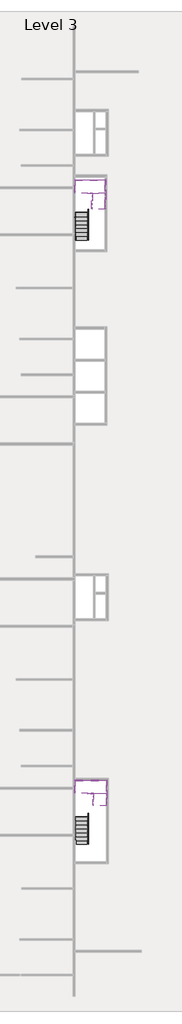
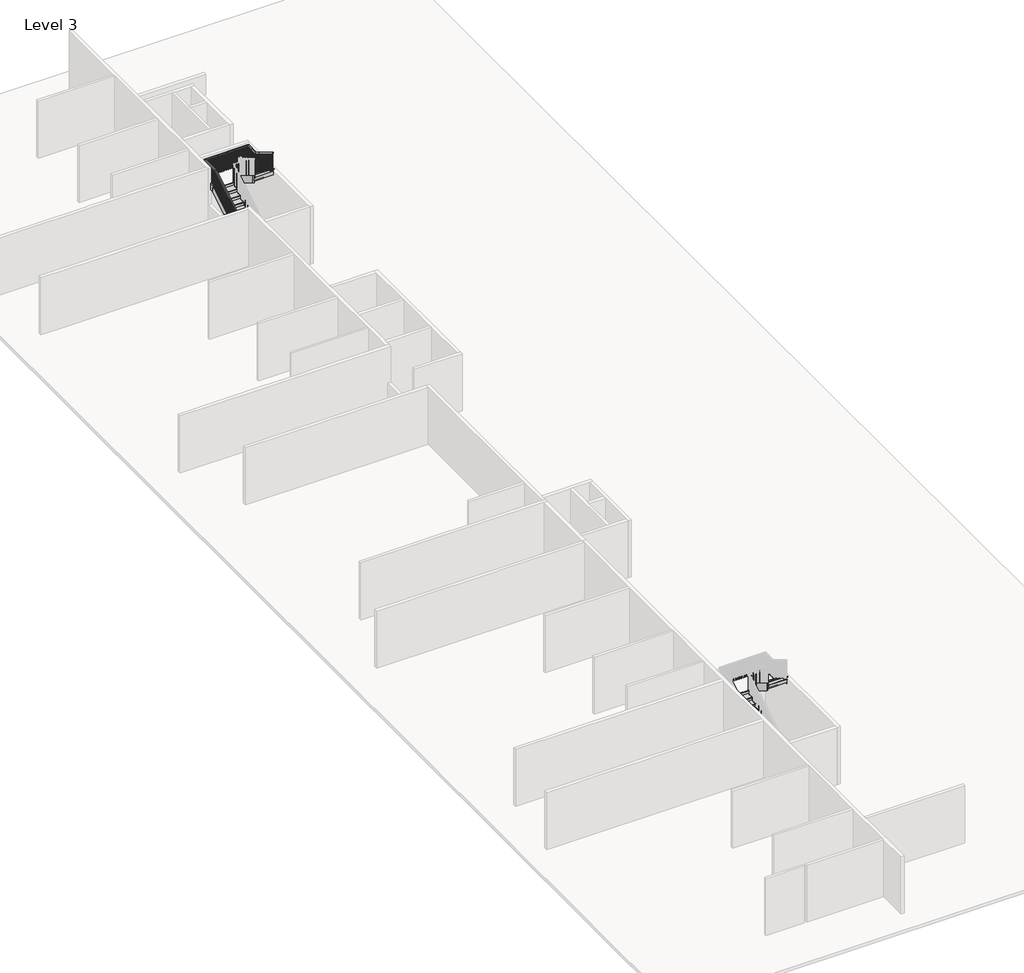
# One storey, part 8 of 8: 16 members, 4 stair flights, 2 slabs, 1 railing.
"""IFC4 building model written with IfcOpenShell, lengths in millimetres."""

from ifc_helpers import new_model, si_unit, frame, origin, place, context, project, spatial, polyline, outline, extrude, faceted_brep, transform, mapped, element, save
from components import non_monolithic_landing_2d4b1833, non_monolithic_landing_0968bfc6, stair_flight_fa816d22, stair_flight_5a0a31fc, stair_flight_0d59740e, stair_flight_4ac50f61

model = new_model("IFC4")

# Units and contexts
model_context = context("Model", 3, world=origin())
ifc_project = project(units=[si_unit("LENGTHUNIT", "METRE", prefix="MILLI")], contexts=[model_context])

# Site, building, storey
site = spatial("IfcSite", under=ifc_project)
building = spatial("IfcBuilding", under=site)
storey = spatial("IfcBuildingStorey", under=building, Name="Level 3", Elevation=31330.6172466)

# Members
placement = place(None, origin())
element("IfcMember", 1, ObjectType="Stringer - 2\" Width", at=placement, inside=storey, context=model_context, shape_type="SweptSolid", body=[
    extrude(outline(polyline([(-23154.3851539, 31330.6172466), (-23154.3851539, 31542.7317586), (-19467.0440987, 33777.4839133), (-19381.8896422, 33472.6839133), (-22916.2996422, 31330.6172466), (-23154.3851539, 31330.6172466)])), frame((-3668.2415084, 0.0, 0.0), z_axis=(1.0, 0.0, 0.0), x_axis=(0.0, 1.0, 0.0)), (0.0, 0.0, 1.0), 50.8),
])
element("IfcMember", 2, ObjectType="Stringer - 2\" Width", at=placement, inside=storey, context=model_context, shape_type="SweptSolid", body=[
    extrude(outline(polyline([(-23154.3851539, 31330.6172466), (-23154.3851539, 31542.7317586), (-19572.9851539, 33713.2772131), (-19572.9851539, 33356.8684516), (-22916.2996422, 31330.6172466), (-23154.3851539, 31330.6172466)])), frame((-2703.0415084, 0.0, 0.0), z_axis=(1.0, 0.0, 0.0), x_axis=(0.0, 1.0, 0.0)), (0.0, 0.0, 1.0), 50.8),
])
element("IfcMember", 3, ObjectType="Stringer - 2\" Width", at=placement, inside=storey, context=model_context, shape_type="SweptSolid", body=[
    extrude(outline(polyline([(-19297.9262092, 33777.4839133), (-19383.0806657, 33472.6839133), (-20360.3851539, 34064.9896637), (-20360.3851539, 34421.3984252), (-19297.9262092, 33777.4839133)])), frame((-1382.2415084, 0.0, 0.0), z_axis=(1.0, 0.0, 0.0), x_axis=(0.0, 1.0, 0.0)), (0.0, 0.0, 1.0), 50.8),
])
element("IfcMember", 4, ObjectType="Stringer - 2\" Width", at=placement, inside=storey, context=model_context, shape_type="SweptSolid", body=[
    extrude(outline(polyline([(-19522.1851539, 33913.3984252), (-19522.1851539, 33556.9896637), (-20360.3851539, 34064.9896637), (-20360.3851539, 34421.3984252), (-19522.1851539, 33913.3984252)])), frame((-2347.4415084, 0.0, 0.0), z_axis=(1.0, 0.0, 0.0), x_axis=(0.0, 1.0, 0.0)), (0.0, 0.0, 1.0), 50.8),
])
element("IfcMember", 5, ObjectType="Stringer - 2\" Width", at=placement, inside=storey, context=model_context, shape_type="Brep", body=[
    faceted_brep([(-1382.2415084, -19297.9262092, 33777.4839133), (-1331.4415084, -19297.9262092, 33777.4839133), (-1331.4415084, -18556.9851539, 33777.4839133), (-1382.2415084, -18607.7851539, 33777.4839133), (-1382.2415084, -19383.0806657, 33472.6839133), (-1382.2415084, -18607.7851539, 33472.6839133), (-1331.4415084, -19383.0806657, 33472.6839133), (-1331.4415084, -18556.9851539, 33472.6839133)], [[[0, 1, 2, 3]], [[4, 0, 3, 5]], [[6, 4, 5, 7]], [[1, 6, 7, 2]], [[1, 0, 4, 6]], [[2, 7, 5, 3]]]),
])
element("IfcMember", 6, ObjectType="Stringer - 2\" Width", at=placement, inside=storey, context=model_context, shape_type="SweptSolid", body=[
    extrude(outline(polyline([(-1331.4415084, -18556.9851539), (-1382.2415084, -18607.7851539), (-3617.4415084, -18607.7851539), (-3668.2415084, -18556.9851539), (-1331.4415084, -18556.9851539)])), frame((0.0, 0.0, 33472.6839133), z_axis=(0.0, 0.0, 1.0), x_axis=(1.0, 0.0, 0.0)), (0.0, 0.0, 1.0), 304.8),
])
element("IfcMember", 7, ObjectType="Stringer - 2\" Width", at=placement, inside=storey, context=model_context, shape_type="Brep", body=[
    faceted_brep([(-3617.4415084, -18607.7851539, 33777.4839133), (-3668.2415084, -18556.9851539, 33777.4839133), (-3668.2415084, -19467.0440987, 33777.4839133), (-3617.4415084, -19467.0440987, 33777.4839133), (-3617.4415084, -18607.7851539, 33472.6839133), (-3617.4415084, -19381.8896422, 33472.6839133), (-3668.2415084, -18556.9851539, 33472.6839133), (-3668.2415084, -19381.8896422, 33472.6839133)], [[[0, 1, 2, 3]], [[4, 0, 3, 5]], [[6, 4, 5, 7]], [[1, 6, 7, 2]], [[1, 0, 4, 6]], [[2, 7, 5, 3]]]),
])
element("IfcMember", 8, ObjectType="Stringer - 2\" Width", at=placement, inside=storey, context=model_context, shape_type="SweptSolid", body=[
    extrude(outline(polyline([(-2703.0415084, -19572.9851539), (-2703.0415084, -19522.1851539), (-2347.4415084, -19522.1851539), (-2347.4415084, -19572.9851539), (-2703.0415084, -19572.9851539)])), frame((0.0, 0.0, 33472.6839133), z_axis=(0.0, 0.0, 1.0), x_axis=(1.0, 0.0, 0.0)), (0.0, 0.0, 1.0), 304.8),
])
element("IfcMember", 9, ObjectType="Stringer - 2\" Width", at=placement, inside=storey, context=model_context, shape_type="SweptSolid", body=[
    extrude(outline(polyline([(19841.9216096, 31330.6172466), (19841.9216096, 31542.7317586), (23249.8626649, 33608.1505799), (23335.0171214, 33303.3505799), (20080.0071214, 31330.6172466), (19841.9216096, 31330.6172466)])), frame((-3668.2415084, 0.0, 0.0), z_axis=(1.0, 0.0, 0.0), x_axis=(0.0, 1.0, 0.0)), (0.0, 0.0, 1.0), 50.8),
])
element("IfcMember", 10, ObjectType="Stringer - 2\" Width", at=placement, inside=storey, context=model_context, shape_type="SweptSolid", body=[
    extrude(outline(polyline([(19841.9216096, 31330.6172466), (19841.9216096, 31542.7317586), (23143.9216096, 33543.9438798), (23143.9216096, 33187.5351183), (20080.0071214, 31330.6172466), (19841.9216096, 31330.6172466)])), frame((-2703.0415084, 0.0, 0.0), z_axis=(1.0, 0.0, 0.0), x_axis=(0.0, 1.0, 0.0)), (0.0, 0.0, 1.0), 50.8),
])
element("IfcMember", 11, ObjectType="Stringer - 2\" Width", at=placement, inside=storey, context=model_context, shape_type="SweptSolid", body=[
    extrude(outline(polyline([(23418.9805543, 33608.1505799), (23333.8260978, 33303.3505799), (22077.1216096, 34064.9896637), (22077.1216096, 34421.3984252), (23418.9805543, 33608.1505799)])), frame((-1483.8415084, 0.0, 0.0), z_axis=(1.0, 0.0, 0.0), x_axis=(0.0, 1.0, 0.0)), (0.0, 0.0, 1.0), 50.8),
])
element("IfcMember", 12, ObjectType="Stringer - 2\" Width", at=placement, inside=storey, context=model_context, shape_type="SweptSolid", body=[
    extrude(outline(polyline([(23194.7216096, 33744.0650919), (23194.7216096, 33387.6563304), (22077.1216096, 34064.9896637), (22077.1216096, 34421.3984252), (23194.7216096, 33744.0650919)])), frame((-2449.0415084, 0.0, 0.0), z_axis=(1.0, 0.0, 0.0), x_axis=(0.0, 1.0, 0.0)), (0.0, 0.0, 1.0), 50.8),
])
element("IfcMember", 13, ObjectType="Stringer - 2\" Width", at=placement, inside=storey, context=model_context, shape_type="Brep", body=[
    faceted_brep([(-1483.8415084, 23418.9805543, 33608.1505799), (-1433.0415084, 23418.9805543, 33608.1505799), (-1433.0415084, 24159.9216096, 33608.1505799), (-1483.8415084, 24109.1216096, 33608.1505799), (-1483.8415084, 23333.8260978, 33303.3505799), (-1483.8415084, 24109.1216096, 33303.3505799), (-1433.0415084, 23333.8260978, 33303.3505799), (-1433.0415084, 24159.9216096, 33303.3505799)], [[[0, 1, 2, 3]], [[4, 0, 3, 5]], [[6, 4, 5, 7]], [[1, 6, 7, 2]], [[1, 0, 4, 6]], [[2, 7, 5, 3]]]),
])
element("IfcMember", 14, ObjectType="Stringer - 2\" Width", at=placement, inside=storey, context=model_context, shape_type="SweptSolid", body=[
    extrude(outline(polyline([(-1433.0415084, 24159.9216096), (-1483.8415084, 24109.1216096), (-3617.4415084, 24109.1216096), (-3668.2415084, 24159.9216096), (-1433.0415084, 24159.9216096)])), frame((0.0, 0.0, 33303.3505799), z_axis=(0.0, 0.0, 1.0), x_axis=(1.0, 0.0, 0.0)), (0.0, 0.0, 1.0), 304.8),
])
element("IfcMember", 15, ObjectType="Stringer - 2\" Width", at=placement, inside=storey, context=model_context, shape_type="Brep", body=[
    faceted_brep([(-3617.4415084, 24109.1216096, 33608.1505799), (-3668.2415084, 24159.9216096, 33608.1505799), (-3668.2415084, 23249.8626649, 33608.1505799), (-3617.4415084, 23249.8626649, 33608.1505799), (-3617.4415084, 24109.1216096, 33303.3505799), (-3617.4415084, 23335.0171214, 33303.3505799), (-3668.2415084, 24159.9216096, 33303.3505799), (-3668.2415084, 23335.0171214, 33303.3505799)], [[[0, 1, 2, 3]], [[4, 0, 3, 5]], [[6, 4, 5, 7]], [[1, 6, 7, 2]], [[1, 0, 4, 6]], [[2, 7, 5, 3]]]),
])
element("IfcMember", 16, ObjectType="Stringer - 2\" Width", at=placement, inside=storey, context=model_context, shape_type="SweptSolid", body=[
    extrude(outline(polyline([(-2703.0415084, 23143.9216096), (-2703.0415084, 23194.7216096), (-2449.0415084, 23194.7216096), (-2449.0415084, 23143.9216096), (-2703.0415084, 23143.9216096)])), frame((0.0, 0.0, 33303.3505799), z_axis=(0.0, 0.0, 1.0), x_axis=(1.0, 0.0, 0.0)), (0.0, 0.0, 1.0), 304.8),
])

# Railing
element("IfcRailing", 17, ObjectType="Handrail - Rectangular", at=placement, inside=storey, context=model_context, shape_type="SolidModel", body=[
    faceted_brep([(-3617.4415084, 19841.9216096, 32414.3505799), (-3617.4415084, 19841.9216096, 32354.9491197), (-3566.6415084, 19841.9216096, 32354.9491197), (-3566.6415084, 19841.9216096, 32414.3505799), (-3617.4415084, 23194.7216096, 34446.3505799), (-3617.4415084, 23208.914019, 34395.5505799), (-3566.6415084, 23208.914019, 34395.5505799), (-3566.6415084, 23194.7216096, 34446.3505799), (-3617.4415084, 24109.1216096, 34446.3505799), (-3617.4415084, 24109.1216096, 34395.5505799), (-3566.6415084, 24058.3216096, 34395.5505799), (-3566.6415084, 24058.3216096, 34446.3505799), (-1483.8415084, 24109.1216096, 34446.3505799), (-1483.8415084, 24109.1216096, 34395.5505799), (-1534.6415084, 24058.3216096, 34395.5505799), (-1534.6415084, 24058.3216096, 34446.3505799), (-1483.8415084, 23474.1216096, 34446.3505799), (-1483.8415084, 23459.9292002, 34395.5505799), (-1534.6415084, 23459.9292002, 34395.5505799), (-1534.6415084, 23474.1216096, 34446.3505799), (-1483.8415084, 23194.7216096, 34615.6839133), (-1483.8415084, 23168.3918824, 34572.2398634), (-1534.6415084, 23168.3918824, 34572.2398634), (-1534.6415084, 23194.7216096, 34615.6839133), (-1483.8415084, 22077.1216096, 35293.0172466), (-1534.6415084, 22077.1216096, 35293.0172466), (-1534.6415084, 22077.1216096, 35233.6157863), (-1483.8415084, 22077.1216096, 35233.6157863)], [[[0, 1, 2, 3]], [[1, 0, 4, 5]], [[2, 1, 5, 6]], [[3, 2, 6, 7]], [[0, 3, 7, 4]], [[5, 4, 8, 9]], [[6, 5, 9, 10]], [[7, 6, 10, 11]], [[4, 7, 11, 8]], [[9, 8, 12, 13]], [[10, 9, 13, 14]], [[11, 10, 14, 15]], [[8, 11, 15, 12]], [[13, 12, 16, 17]], [[14, 13, 17, 18]], [[15, 14, 18, 19]], [[12, 15, 19, 16]], [[17, 16, 20, 21]], [[18, 17, 21, 22]], [[19, 18, 22, 23]], [[16, 19, 23, 20]], [[24, 25, 26, 27]], [[21, 20, 24, 27]], [[22, 21, 27, 26]], [[23, 22, 26, 25]], [[20, 23, 25, 24]]]),
    extrude(outline(polyline([(22188.2466096, 35166.2673015), (22188.2466096, 34209.2839133), (22169.1966096, 34209.2839133), (22169.1966096, 35177.812756), (22188.2466096, 35166.2673015)])), frame((-1518.7665084, 0.0, 0.0), z_axis=(1.0, 0.0, 0.0), x_axis=(0.0, 1.0, 0.0)), (0.0, 0.0, 1.0), 19.05),
    extrude(outline(polyline([(22289.8466096, 35104.6915439), (22289.8466096, 34209.2839133), (22270.7966096, 34209.2839133), (22270.7966096, 35116.2369985), (22289.8466096, 35104.6915439)])), frame((-1518.7665084, 0.0, 0.0), z_axis=(1.0, 0.0, 0.0), x_axis=(0.0, 1.0, 0.0)), (0.0, 0.0, 1.0), 19.05),
    extrude(outline(polyline([(22391.4466096, 35043.1157863), (22391.4466096, 34039.9505799), (22372.3966096, 34039.9505799), (22372.3966096, 35054.6612409), (22391.4466096, 35043.1157863)])), frame((-1518.7665084, 0.0, 0.0), z_axis=(1.0, 0.0, 0.0), x_axis=(0.0, 1.0, 0.0)), (0.0, 0.0, 1.0), 19.05),
    extrude(outline(polyline([(22493.0466096, 34981.5400288), (22493.0466096, 34039.9505799), (22473.9966096, 34039.9505799), (22473.9966096, 34993.0854833), (22493.0466096, 34981.5400288)])), frame((-1518.7665084, 0.0, 0.0), z_axis=(1.0, 0.0, 0.0), x_axis=(0.0, 1.0, 0.0)), (0.0, 0.0, 1.0), 19.05),
    extrude(outline(polyline([(22594.6466096, 34919.9642712), (22594.6466096, 34039.9505799), (22575.5966096, 34039.9505799), (22575.5966096, 34931.5097257), (22594.6466096, 34919.9642712)])), frame((-1518.7665084, 0.0, 0.0), z_axis=(1.0, 0.0, 0.0), x_axis=(0.0, 1.0, 0.0)), (0.0, 0.0, 1.0), 19.05),
    extrude(outline(polyline([(22696.2466096, 34858.3885136), (22696.2466096, 33870.6172466), (22677.1966096, 33870.6172466), (22677.1966096, 34869.9339682), (22696.2466096, 34858.3885136)])), frame((-1518.7665084, 0.0, 0.0), z_axis=(1.0, 0.0, 0.0), x_axis=(0.0, 1.0, 0.0)), (0.0, 0.0, 1.0), 19.05),
    extrude(outline(polyline([(22797.8466096, 34796.812756), (22797.8466096, 33870.6172466), (22778.7966096, 33870.6172466), (22778.7966096, 34808.3582106), (22797.8466096, 34796.812756)])), frame((-1518.7665084, 0.0, 0.0), z_axis=(1.0, 0.0, 0.0), x_axis=(0.0, 1.0, 0.0)), (0.0, 0.0, 1.0), 19.05),
    extrude(outline(polyline([(22899.4466096, 34735.2369985), (22899.4466096, 33870.6172466), (22880.3966096, 33870.6172466), (22880.3966096, 34746.782453), (22899.4466096, 34735.2369985)])), frame((-1518.7665084, 0.0, 0.0), z_axis=(1.0, 0.0, 0.0), x_axis=(0.0, 1.0, 0.0)), (0.0, 0.0, 1.0), 19.05),
    extrude(outline(polyline([(23001.0466096, 34673.6612409), (23001.0466096, 33701.2839133), (22981.9966096, 33701.2839133), (22981.9966096, 34685.2066954), (23001.0466096, 34673.6612409)])), frame((-1518.7665084, 0.0, 0.0), z_axis=(1.0, 0.0, 0.0), x_axis=(0.0, 1.0, 0.0)), (0.0, 0.0, 1.0), 19.05),
    extrude(outline(polyline([(23102.6466096, 34612.0854833), (23102.6466096, 33701.2839133), (23083.5966096, 33701.2839133), (23083.5966096, 34623.6309379), (23102.6466096, 34612.0854833)])), frame((-1518.7665084, 0.0, 0.0), z_axis=(1.0, 0.0, 0.0), x_axis=(0.0, 1.0, 0.0)), (0.0, 0.0, 1.0), 19.05),
    extrude(outline(polyline([(23280.4466096, 34504.3279076), (23280.4466096, 33531.9505799), (23261.3966096, 33531.9505799), (23261.3966096, 34515.8733621), (23280.4466096, 34504.3279076)])), frame((-1518.7665084, 0.0, 0.0), z_axis=(1.0, 0.0, 0.0), x_axis=(0.0, 1.0, 0.0)), (0.0, 0.0, 1.0), 19.05),
    extrude(outline(polyline([(23382.0466096, 34442.75215), (23382.0466096, 33531.9505799), (23362.9966096, 33531.9505799), (23362.9966096, 34454.2976045), (23382.0466096, 34442.75215)])), frame((-1518.7665084, 0.0, 0.0), z_axis=(1.0, 0.0, 0.0), x_axis=(0.0, 1.0, 0.0)), (0.0, 0.0, 1.0), 19.05),
    extrude(outline(polyline([(-1499.7165084, 23483.6466096), (-1499.7165084, 23464.5966096), (-1518.7665084, 23464.5966096), (-1518.7665084, 23483.6466096), (-1499.7165084, 23483.6466096)])), frame((0.0, 0.0, 33531.9505799), z_axis=(0.0, 0.0, 1.0), x_axis=(1.0, 0.0, 0.0)), (0.0, 0.0, 1.0), 863.6),
    extrude(outline(polyline([(-1499.7165084, 23585.2466096), (-1499.7165084, 23566.1966096), (-1518.7665084, 23566.1966096), (-1518.7665084, 23585.2466096), (-1499.7165084, 23585.2466096)])), frame((0.0, 0.0, 33531.9505799), z_axis=(0.0, 0.0, 1.0), x_axis=(1.0, 0.0, 0.0)), (0.0, 0.0, 1.0), 863.6),
    extrude(outline(polyline([(-1499.7165084, 23686.8466096), (-1499.7165084, 23667.7966096), (-1518.7665084, 23667.7966096), (-1518.7665084, 23686.8466096), (-1499.7165084, 23686.8466096)])), frame((0.0, 0.0, 33531.9505799), z_axis=(0.0, 0.0, 1.0), x_axis=(1.0, 0.0, 0.0)), (0.0, 0.0, 1.0), 863.6),
    extrude(outline(polyline([(-1499.7165084, 23788.4466096), (-1499.7165084, 23769.3966096), (-1518.7665084, 23769.3966096), (-1518.7665084, 23788.4466096), (-1499.7165084, 23788.4466096)])), frame((0.0, 0.0, 33531.9505799), z_axis=(0.0, 0.0, 1.0), x_axis=(1.0, 0.0, 0.0)), (0.0, 0.0, 1.0), 863.6),
    extrude(outline(polyline([(-1499.7165084, 23890.0466096), (-1499.7165084, 23870.9966096), (-1518.7665084, 23870.9966096), (-1518.7665084, 23890.0466096), (-1499.7165084, 23890.0466096)])), frame((0.0, 0.0, 33531.9505799), z_axis=(0.0, 0.0, 1.0), x_axis=(1.0, 0.0, 0.0)), (0.0, 0.0, 1.0), 863.6),
    extrude(outline(polyline([(-1499.7165084, 23991.6466096), (-1499.7165084, 23972.5966096), (-1518.7665084, 23972.5966096), (-1518.7665084, 23991.6466096), (-1499.7165084, 23991.6466096)])), frame((0.0, 0.0, 33531.9505799), z_axis=(0.0, 0.0, 1.0), x_axis=(1.0, 0.0, 0.0)), (0.0, 0.0, 1.0), 863.6),
    extrude(outline(polyline([(-1569.5665084, 24093.2466096), (-1550.5165084, 24093.2466096), (-1550.5165084, 24074.1966096), (-1569.5665084, 24074.1966096), (-1569.5665084, 24093.2466096)])), frame((0.0, 0.0, 33531.9505799), z_axis=(0.0, 0.0, 1.0), x_axis=(1.0, 0.0, 0.0)), (0.0, 0.0, 1.0), 863.6),
    extrude(outline(polyline([(-1671.1665084, 24093.2466096), (-1652.1165084, 24093.2466096), (-1652.1165084, 24074.1966096), (-1671.1665084, 24074.1966096), (-1671.1665084, 24093.2466096)])), frame((0.0, 0.0, 33531.9505799), z_axis=(0.0, 0.0, 1.0), x_axis=(1.0, 0.0, 0.0)), (0.0, 0.0, 1.0), 863.6),
    extrude(outline(polyline([(-1772.7665084, 24093.2466096), (-1753.7165084, 24093.2466096), (-1753.7165084, 24074.1966096), (-1772.7665084, 24074.1966096), (-1772.7665084, 24093.2466096)])), frame((0.0, 0.0, 33531.9505799), z_axis=(0.0, 0.0, 1.0), x_axis=(1.0, 0.0, 0.0)), (0.0, 0.0, 1.0), 863.6),
    extrude(outline(polyline([(-1874.3665084, 24093.2466096), (-1855.3165084, 24093.2466096), (-1855.3165084, 24074.1966096), (-1874.3665084, 24074.1966096), (-1874.3665084, 24093.2466096)])), frame((0.0, 0.0, 33531.9505799), z_axis=(0.0, 0.0, 1.0), x_axis=(1.0, 0.0, 0.0)), (0.0, 0.0, 1.0), 863.6),
    extrude(outline(polyline([(-1975.9665084, 24093.2466096), (-1956.9165084, 24093.2466096), (-1956.9165084, 24074.1966096), (-1975.9665084, 24074.1966096), (-1975.9665084, 24093.2466096)])), frame((0.0, 0.0, 33531.9505799), z_axis=(0.0, 0.0, 1.0), x_axis=(1.0, 0.0, 0.0)), (0.0, 0.0, 1.0), 863.6),
    extrude(outline(polyline([(-2077.5665084, 24093.2466096), (-2058.5165084, 24093.2466096), (-2058.5165084, 24074.1966096), (-2077.5665084, 24074.1966096), (-2077.5665084, 24093.2466096)])), frame((0.0, 0.0, 33531.9505799), z_axis=(0.0, 0.0, 1.0), x_axis=(1.0, 0.0, 0.0)), (0.0, 0.0, 1.0), 863.6),
    extrude(outline(polyline([(-2179.1665084, 24093.2466096), (-2160.1165084, 24093.2466096), (-2160.1165084, 24074.1966096), (-2179.1665084, 24074.1966096), (-2179.1665084, 24093.2466096)])), frame((0.0, 0.0, 33531.9505799), z_axis=(0.0, 0.0, 1.0), x_axis=(1.0, 0.0, 0.0)), (0.0, 0.0, 1.0), 863.6),
    extrude(outline(polyline([(-2280.7665084, 24093.2466096), (-2261.7165084, 24093.2466096), (-2261.7165084, 24074.1966096), (-2280.7665084, 24074.1966096), (-2280.7665084, 24093.2466096)])), frame((0.0, 0.0, 33531.9505799), z_axis=(0.0, 0.0, 1.0), x_axis=(1.0, 0.0, 0.0)), (0.0, 0.0, 1.0), 863.6),
    extrude(outline(polyline([(-2382.3665084, 24093.2466096), (-2363.3165084, 24093.2466096), (-2363.3165084, 24074.1966096), (-2382.3665084, 24074.1966096), (-2382.3665084, 24093.2466096)])), frame((0.0, 0.0, 33531.9505799), z_axis=(0.0, 0.0, 1.0), x_axis=(1.0, 0.0, 0.0)), (0.0, 0.0, 1.0), 863.6),
    extrude(outline(polyline([(-2483.9665084, 24093.2466096), (-2464.9165084, 24093.2466096), (-2464.9165084, 24074.1966096), (-2483.9665084, 24074.1966096), (-2483.9665084, 24093.2466096)])), frame((0.0, 0.0, 33531.9505799), z_axis=(0.0, 0.0, 1.0), x_axis=(1.0, 0.0, 0.0)), (0.0, 0.0, 1.0), 863.6),
    extrude(outline(polyline([(-2585.5665084, 24093.2466096), (-2566.5165084, 24093.2466096), (-2566.5165084, 24074.1966096), (-2585.5665084, 24074.1966096), (-2585.5665084, 24093.2466096)])), frame((0.0, 0.0, 33531.9505799), z_axis=(0.0, 0.0, 1.0), x_axis=(1.0, 0.0, 0.0)), (0.0, 0.0, 1.0), 863.6),
    extrude(outline(polyline([(-2687.1665084, 24093.2466096), (-2668.1165084, 24093.2466096), (-2668.1165084, 24074.1966096), (-2687.1665084, 24074.1966096), (-2687.1665084, 24093.2466096)])), frame((0.0, 0.0, 33531.9505799), z_axis=(0.0, 0.0, 1.0), x_axis=(1.0, 0.0, 0.0)), (0.0, 0.0, 1.0), 863.6),
    extrude(outline(polyline([(-2788.7665084, 24093.2466096), (-2769.7165084, 24093.2466096), (-2769.7165084, 24074.1966096), (-2788.7665084, 24074.1966096), (-2788.7665084, 24093.2466096)])), frame((0.0, 0.0, 33531.9505799), z_axis=(0.0, 0.0, 1.0), x_axis=(1.0, 0.0, 0.0)), (0.0, 0.0, 1.0), 863.6),
    extrude(outline(polyline([(-2890.3665084, 24093.2466096), (-2871.3165084, 24093.2466096), (-2871.3165084, 24074.1966096), (-2890.3665084, 24074.1966096), (-2890.3665084, 24093.2466096)])), frame((0.0, 0.0, 33531.9505799), z_axis=(0.0, 0.0, 1.0), x_axis=(1.0, 0.0, 0.0)), (0.0, 0.0, 1.0), 863.6),
    extrude(outline(polyline([(-2991.9665084, 24093.2466096), (-2972.9165084, 24093.2466096), (-2972.9165084, 24074.1966096), (-2991.9665084, 24074.1966096), (-2991.9665084, 24093.2466096)])), frame((0.0, 0.0, 33531.9505799), z_axis=(0.0, 0.0, 1.0), x_axis=(1.0, 0.0, 0.0)), (0.0, 0.0, 1.0), 863.6),
    extrude(outline(polyline([(-3093.5665084, 24093.2466096), (-3074.5165084, 24093.2466096), (-3074.5165084, 24074.1966096), (-3093.5665084, 24074.1966096), (-3093.5665084, 24093.2466096)])), frame((0.0, 0.0, 33531.9505799), z_axis=(0.0, 0.0, 1.0), x_axis=(1.0, 0.0, 0.0)), (0.0, 0.0, 1.0), 863.6),
    extrude(outline(polyline([(-3195.1665084, 24093.2466096), (-3176.1165084, 24093.2466096), (-3176.1165084, 24074.1966096), (-3195.1665084, 24074.1966096), (-3195.1665084, 24093.2466096)])), frame((0.0, 0.0, 33531.9505799), z_axis=(0.0, 0.0, 1.0), x_axis=(1.0, 0.0, 0.0)), (0.0, 0.0, 1.0), 863.6),
    extrude(outline(polyline([(-3296.7665084, 24093.2466096), (-3277.7165084, 24093.2466096), (-3277.7165084, 24074.1966096), (-3296.7665084, 24074.1966096), (-3296.7665084, 24093.2466096)])), frame((0.0, 0.0, 33531.9505799), z_axis=(0.0, 0.0, 1.0), x_axis=(1.0, 0.0, 0.0)), (0.0, 0.0, 1.0), 863.6),
    extrude(outline(polyline([(-3398.3665084, 24093.2466096), (-3379.3165084, 24093.2466096), (-3379.3165084, 24074.1966096), (-3398.3665084, 24074.1966096), (-3398.3665084, 24093.2466096)])), frame((0.0, 0.0, 33531.9505799), z_axis=(0.0, 0.0, 1.0), x_axis=(1.0, 0.0, 0.0)), (0.0, 0.0, 1.0), 863.6),
    extrude(outline(polyline([(-3499.9665084, 24093.2466096), (-3480.9165084, 24093.2466096), (-3480.9165084, 24074.1966096), (-3499.9665084, 24074.1966096), (-3499.9665084, 24093.2466096)])), frame((0.0, 0.0, 33531.9505799), z_axis=(0.0, 0.0, 1.0), x_axis=(1.0, 0.0, 0.0)), (0.0, 0.0, 1.0), 863.6),
    extrude(outline(polyline([(-3601.5665084, 23997.9966096), (-3601.5665084, 24017.0466096), (-3582.5165084, 24017.0466096), (-3582.5165084, 23997.9966096), (-3601.5665084, 23997.9966096)])), frame((0.0, 0.0, 33531.9505799), z_axis=(0.0, 0.0, 1.0), x_axis=(1.0, 0.0, 0.0)), (0.0, 0.0, 1.0), 863.6),
    extrude(outline(polyline([(-3601.5665084, 23896.3966096), (-3601.5665084, 23915.4466096), (-3582.5165084, 23915.4466096), (-3582.5165084, 23896.3966096), (-3601.5665084, 23896.3966096)])), frame((0.0, 0.0, 33531.9505799), z_axis=(0.0, 0.0, 1.0), x_axis=(1.0, 0.0, 0.0)), (0.0, 0.0, 1.0), 863.6),
    extrude(outline(polyline([(-3601.5665084, 23794.7966096), (-3601.5665084, 23813.8466096), (-3582.5165084, 23813.8466096), (-3582.5165084, 23794.7966096), (-3601.5665084, 23794.7966096)])), frame((0.0, 0.0, 33531.9505799), z_axis=(0.0, 0.0, 1.0), x_axis=(1.0, 0.0, 0.0)), (0.0, 0.0, 1.0), 863.6),
    extrude(outline(polyline([(-3601.5665084, 23693.1966096), (-3601.5665084, 23712.2466096), (-3582.5165084, 23712.2466096), (-3582.5165084, 23693.1966096), (-3601.5665084, 23693.1966096)])), frame((0.0, 0.0, 33531.9505799), z_axis=(0.0, 0.0, 1.0), x_axis=(1.0, 0.0, 0.0)), (0.0, 0.0, 1.0), 863.6),
    extrude(outline(polyline([(-3601.5665084, 23591.5966096), (-3601.5665084, 23610.6466096), (-3582.5165084, 23610.6466096), (-3582.5165084, 23591.5966096), (-3601.5665084, 23591.5966096)])), frame((0.0, 0.0, 33531.9505799), z_axis=(0.0, 0.0, 1.0), x_axis=(1.0, 0.0, 0.0)), (0.0, 0.0, 1.0), 863.6),
    extrude(outline(polyline([(-3601.5665084, 23489.9966096), (-3601.5665084, 23509.0466096), (-3582.5165084, 23509.0466096), (-3582.5165084, 23489.9966096), (-3601.5665084, 23489.9966096)])), frame((0.0, 0.0, 33531.9505799), z_axis=(0.0, 0.0, 1.0), x_axis=(1.0, 0.0, 0.0)), (0.0, 0.0, 1.0), 863.6),
    extrude(outline(polyline([(-3601.5665084, 23388.3966096), (-3601.5665084, 23407.4466096), (-3582.5165084, 23407.4466096), (-3582.5165084, 23388.3966096), (-3601.5665084, 23388.3966096)])), frame((0.0, 0.0, 33531.9505799), z_axis=(0.0, 0.0, 1.0), x_axis=(1.0, 0.0, 0.0)), (0.0, 0.0, 1.0), 863.6),
    extrude(outline(polyline([(-3601.5665084, 23286.7966096), (-3601.5665084, 23305.8466096), (-3582.5165084, 23305.8466096), (-3582.5165084, 23286.7966096), (-3601.5665084, 23286.7966096)])), frame((0.0, 0.0, 33531.9505799), z_axis=(0.0, 0.0, 1.0), x_axis=(1.0, 0.0, 0.0)), (0.0, 0.0, 1.0), 863.6),
    extrude(outline(polyline([(23102.6466096, 34331.1460894), (23102.6466096, 33362.6172466), (23083.5966096, 33362.6172466), (23083.5966096, 34319.6006348), (23102.6466096, 34331.1460894)])), frame((-3601.5665084, 0.0, 0.0), z_axis=(1.0, 0.0, 0.0), x_axis=(0.0, 1.0, 0.0)), (0.0, 0.0, 1.0), 19.05),
    extrude(outline(polyline([(23001.0466096, 34269.5703318), (23001.0466096, 33362.6172466), (22981.9966096, 33362.6172466), (22981.9966096, 34258.0248773), (23001.0466096, 34269.5703318)])), frame((-3601.5665084, 0.0, 0.0), z_axis=(1.0, 0.0, 0.0), x_axis=(0.0, 1.0, 0.0)), (0.0, 0.0, 1.0), 19.05),
    extrude(outline(polyline([(22899.4466096, 34207.9945742), (22899.4466096, 33193.2839133), (22880.3966096, 33193.2839133), (22880.3966096, 34196.4491197), (22899.4466096, 34207.9945742)])), frame((-3601.5665084, 0.0, 0.0), z_axis=(1.0, 0.0, 0.0), x_axis=(0.0, 1.0, 0.0)), (0.0, 0.0, 1.0), 19.05),
    extrude(outline(polyline([(22797.8466096, 34146.4188166), (22797.8466096, 33193.2839133), (22778.7966096, 33193.2839133), (22778.7966096, 34134.8733621), (22797.8466096, 34146.4188166)])), frame((-3601.5665084, 0.0, 0.0), z_axis=(1.0, 0.0, 0.0), x_axis=(0.0, 1.0, 0.0)), (0.0, 0.0, 1.0), 19.05),
    extrude(outline(polyline([(22696.2466096, 34084.8430591), (22696.2466096, 33193.2839133), (22677.1966096, 33193.2839133), (22677.1966096, 34073.2976045), (22696.2466096, 34084.8430591)])), frame((-3601.5665084, 0.0, 0.0), z_axis=(1.0, 0.0, 0.0), x_axis=(0.0, 1.0, 0.0)), (0.0, 0.0, 1.0), 19.05),
    extrude(outline(polyline([(22594.6466096, 34023.2673015), (22594.6466096, 33023.9505799), (22575.5966096, 33023.9505799), (22575.5966096, 34011.721847), (22594.6466096, 34023.2673015)])), frame((-3601.5665084, 0.0, 0.0), z_axis=(1.0, 0.0, 0.0), x_axis=(0.0, 1.0, 0.0)), (0.0, 0.0, 1.0), 19.05),
    extrude(outline(polyline([(22493.0466096, 33961.6915439), (22493.0466096, 33023.9505799), (22473.9966096, 33023.9505799), (22473.9966096, 33950.1460894), (22493.0466096, 33961.6915439)])), frame((-3601.5665084, 0.0, 0.0), z_axis=(1.0, 0.0, 0.0), x_axis=(0.0, 1.0, 0.0)), (0.0, 0.0, 1.0), 19.05),
    extrude(outline(polyline([(22391.4466096, 33900.1157863), (22391.4466096, 33023.9505799), (22372.3966096, 33023.9505799), (22372.3966096, 33888.5703318), (22391.4466096, 33900.1157863)])), frame((-3601.5665084, 0.0, 0.0), z_axis=(1.0, 0.0, 0.0), x_axis=(0.0, 1.0, 0.0)), (0.0, 0.0, 1.0), 19.05),
    extrude(outline(polyline([(22289.8466096, 33838.5400288), (22289.8466096, 32854.6172466), (22270.7966096, 32854.6172466), (22270.7966096, 33826.9945742), (22289.8466096, 33838.5400288)])), frame((-3601.5665084, 0.0, 0.0), z_axis=(1.0, 0.0, 0.0), x_axis=(0.0, 1.0, 0.0)), (0.0, 0.0, 1.0), 19.05),
    extrude(outline(polyline([(22188.2466096, 33776.9642712), (22188.2466096, 32854.6172466), (22169.1966096, 32854.6172466), (22169.1966096, 33765.4188166), (22188.2466096, 33776.9642712)])), frame((-3601.5665084, 0.0, 0.0), z_axis=(1.0, 0.0, 0.0), x_axis=(0.0, 1.0, 0.0)), (0.0, 0.0, 1.0), 19.05),
    extrude(outline(polyline([(22086.6466096, 33715.3885136), (22086.6466096, 32854.6172466), (22067.5966096, 32854.6172466), (22067.5966096, 33703.8430591), (22086.6466096, 33715.3885136)])), frame((-3601.5665084, 0.0, 0.0), z_axis=(1.0, 0.0, 0.0), x_axis=(0.0, 1.0, 0.0)), (0.0, 0.0, 1.0), 19.05),
    extrude(outline(polyline([(21985.0466096, 33653.812756), (21985.0466096, 32685.2839133), (21965.9966096, 32685.2839133), (21965.9966096, 33642.2673015), (21985.0466096, 33653.812756)])), frame((-3601.5665084, 0.0, 0.0), z_axis=(1.0, 0.0, 0.0), x_axis=(0.0, 1.0, 0.0)), (0.0, 0.0, 1.0), 19.05),
    extrude(outline(polyline([(21883.4466096, 33592.2369985), (21883.4466096, 32685.2839133), (21864.3966096, 32685.2839133), (21864.3966096, 33580.6915439), (21883.4466096, 33592.2369985)])), frame((-3601.5665084, 0.0, 0.0), z_axis=(1.0, 0.0, 0.0), x_axis=(0.0, 1.0, 0.0)), (0.0, 0.0, 1.0), 19.05),
    extrude(outline(polyline([(21781.8466096, 33530.6612409), (21781.8466096, 32515.9505799), (21762.7966096, 32515.9505799), (21762.7966096, 33519.1157863), (21781.8466096, 33530.6612409)])), frame((-3601.5665084, 0.0, 0.0), z_axis=(1.0, 0.0, 0.0), x_axis=(0.0, 1.0, 0.0)), (0.0, 0.0, 1.0), 19.05),
    extrude(outline(polyline([(21680.2466096, 33469.0854833), (21680.2466096, 32515.9505799), (21661.1966096, 32515.9505799), (21661.1966096, 33457.5400288), (21680.2466096, 33469.0854833)])), frame((-3601.5665084, 0.0, 0.0), z_axis=(1.0, 0.0, 0.0), x_axis=(0.0, 1.0, 0.0)), (0.0, 0.0, 1.0), 19.05),
    extrude(outline(polyline([(21578.6466096, 33407.5097257), (21578.6466096, 32515.9505799), (21559.5966096, 32515.9505799), (21559.5966096, 33395.9642712), (21578.6466096, 33407.5097257)])), frame((-3601.5665084, 0.0, 0.0), z_axis=(1.0, 0.0, 0.0), x_axis=(0.0, 1.0, 0.0)), (0.0, 0.0, 1.0), 19.05),
    extrude(outline(polyline([(21477.0466096, 33345.9339682), (21477.0466096, 32346.6172466), (21457.9966096, 32346.6172466), (21457.9966096, 33334.3885136), (21477.0466096, 33345.9339682)])), frame((-3601.5665084, 0.0, 0.0), z_axis=(1.0, 0.0, 0.0), x_axis=(0.0, 1.0, 0.0)), (0.0, 0.0, 1.0), 19.05),
    extrude(outline(polyline([(21375.4466096, 33284.3582106), (21375.4466096, 32346.6172466), (21356.3966096, 32346.6172466), (21356.3966096, 33272.812756), (21375.4466096, 33284.3582106)])), frame((-3601.5665084, 0.0, 0.0), z_axis=(1.0, 0.0, 0.0), x_axis=(0.0, 1.0, 0.0)), (0.0, 0.0, 1.0), 19.05),
    extrude(outline(polyline([(21273.8466096, 33222.782453), (21273.8466096, 32346.6172466), (21254.7966096, 32346.6172466), (21254.7966096, 33211.2369985), (21273.8466096, 33222.782453)])), frame((-3601.5665084, 0.0, 0.0), z_axis=(1.0, 0.0, 0.0), x_axis=(0.0, 1.0, 0.0)), (0.0, 0.0, 1.0), 19.05),
    extrude(outline(polyline([(21172.2466096, 33161.2066954), (21172.2466096, 32177.2839133), (21153.1966096, 32177.2839133), (21153.1966096, 33149.6612409), (21172.2466096, 33161.2066954)])), frame((-3601.5665084, 0.0, 0.0), z_axis=(1.0, 0.0, 0.0), x_axis=(0.0, 1.0, 0.0)), (0.0, 0.0, 1.0), 19.05),
    extrude(outline(polyline([(21070.6466096, 33099.6309379), (21070.6466096, 32177.2839133), (21051.5966096, 32177.2839133), (21051.5966096, 33088.0854833), (21070.6466096, 33099.6309379)])), frame((-3601.5665084, 0.0, 0.0), z_axis=(1.0, 0.0, 0.0), x_axis=(0.0, 1.0, 0.0)), (0.0, 0.0, 1.0), 19.05),
    extrude(outline(polyline([(20969.0466096, 33038.0551803), (20969.0466096, 32177.2839133), (20949.9966096, 32177.2839133), (20949.9966096, 33026.5097257), (20969.0466096, 33038.0551803)])), frame((-3601.5665084, 0.0, 0.0), z_axis=(1.0, 0.0, 0.0), x_axis=(0.0, 1.0, 0.0)), (0.0, 0.0, 1.0), 19.05),
    extrude(outline(polyline([(20867.4466096, 32976.4794227), (20867.4466096, 32007.9505799), (20848.3966096, 32007.9505799), (20848.3966096, 32964.9339682), (20867.4466096, 32976.4794227)])), frame((-3601.5665084, 0.0, 0.0), z_axis=(1.0, 0.0, 0.0), x_axis=(0.0, 1.0, 0.0)), (0.0, 0.0, 1.0), 19.05),
    extrude(outline(polyline([(20765.8466096, 32914.9036651), (20765.8466096, 32007.9505799), (20746.7966096, 32007.9505799), (20746.7966096, 32903.3582106), (20765.8466096, 32914.9036651)])), frame((-3601.5665084, 0.0, 0.0), z_axis=(1.0, 0.0, 0.0), x_axis=(0.0, 1.0, 0.0)), (0.0, 0.0, 1.0), 19.05),
    extrude(outline(polyline([(20664.2466096, 32853.3279076), (20664.2466096, 31838.6172466), (20645.1966096, 31838.6172466), (20645.1966096, 32841.782453), (20664.2466096, 32853.3279076)])), frame((-3601.5665084, 0.0, 0.0), z_axis=(1.0, 0.0, 0.0), x_axis=(0.0, 1.0, 0.0)), (0.0, 0.0, 1.0), 19.05),
    extrude(outline(polyline([(20562.6466096, 32791.75215), (20562.6466096, 31838.6172466), (20543.5966096, 31838.6172466), (20543.5966096, 32780.2066954), (20562.6466096, 32791.75215)])), frame((-3601.5665084, 0.0, 0.0), z_axis=(1.0, 0.0, 0.0), x_axis=(0.0, 1.0, 0.0)), (0.0, 0.0, 1.0), 19.05),
    extrude(outline(polyline([(20461.0466096, 32730.1763924), (20461.0466096, 31838.6172466), (20441.9966096, 31838.6172466), (20441.9966096, 32718.6309379), (20461.0466096, 32730.1763924)])), frame((-3601.5665084, 0.0, 0.0), z_axis=(1.0, 0.0, 0.0), x_axis=(0.0, 1.0, 0.0)), (0.0, 0.0, 1.0), 19.05),
    extrude(outline(polyline([(20359.4466096, 32668.6006348), (20359.4466096, 31669.2839133), (20340.3966096, 31669.2839133), (20340.3966096, 32657.0551803), (20359.4466096, 32668.6006348)])), frame((-3601.5665084, 0.0, 0.0), z_axis=(1.0, 0.0, 0.0), x_axis=(0.0, 1.0, 0.0)), (0.0, 0.0, 1.0), 19.05),
    extrude(outline(polyline([(20257.8466096, 32607.0248773), (20257.8466096, 31669.2839133), (20238.7966096, 31669.2839133), (20238.7966096, 32595.4794227), (20257.8466096, 32607.0248773)])), frame((-3601.5665084, 0.0, 0.0), z_axis=(1.0, 0.0, 0.0), x_axis=(0.0, 1.0, 0.0)), (0.0, 0.0, 1.0), 19.05),
    extrude(outline(polyline([(20156.2466096, 32545.4491197), (20156.2466096, 31669.2839133), (20137.1966096, 31669.2839133), (20137.1966096, 32533.9036651), (20156.2466096, 32545.4491197)])), frame((-3601.5665084, 0.0, 0.0), z_axis=(1.0, 0.0, 0.0), x_axis=(0.0, 1.0, 0.0)), (0.0, 0.0, 1.0), 19.05),
    extrude(outline(polyline([(20054.6466096, 32483.8733621), (20054.6466096, 31499.9505799), (20035.5966096, 31499.9505799), (20035.5966096, 32472.3279076), (20054.6466096, 32483.8733621)])), frame((-3601.5665084, 0.0, 0.0), z_axis=(1.0, 0.0, 0.0), x_axis=(0.0, 1.0, 0.0)), (0.0, 0.0, 1.0), 19.05),
    extrude(outline(polyline([(19953.0466096, 32422.2976045), (19953.0466096, 31499.9505799), (19933.9966096, 31499.9505799), (19933.9966096, 32410.75215), (19953.0466096, 32422.2976045)])), frame((-3601.5665084, 0.0, 0.0), z_axis=(1.0, 0.0, 0.0), x_axis=(0.0, 1.0, 0.0)), (0.0, 0.0, 1.0), 19.05),
    extrude(outline(polyline([(23204.2466096, 34550.5097257), (23204.2466096, 33531.9505799), (23185.1966096, 33531.9505799), (23185.1966096, 34562.0551803), (23204.2466096, 34550.5097257)])), frame((-1518.7665084, 0.0, 0.0), z_axis=(1.0, 0.0, 0.0), x_axis=(0.0, 1.0, 0.0)), (0.0, 0.0, 1.0), 19.05),
    extrude(outline(polyline([(-1518.7665084, 24093.2466096), (-1499.7165084, 24093.2466096), (-1499.7165084, 24074.1966096), (-1518.7665084, 24074.1966096), (-1518.7665084, 24093.2466096)])), frame((0.0, 0.0, 33531.9505799), z_axis=(0.0, 0.0, 1.0), x_axis=(1.0, 0.0, 0.0)), (0.0, 0.0, 1.0), 863.6),
    extrude(outline(polyline([(-3601.5665084, 24074.1966096), (-3601.5665084, 24093.2466096), (-3582.5165084, 24093.2466096), (-3582.5165084, 24074.1966096), (-3601.5665084, 24074.1966096)])), frame((0.0, 0.0, 33531.9505799), z_axis=(0.0, 0.0, 1.0), x_axis=(1.0, 0.0, 0.0)), (0.0, 0.0, 1.0), 863.6),
    extrude(outline(polyline([(23204.2466096, 34392.721847), (23204.2466096, 33531.9505799), (23185.1966096, 33531.9505799), (23185.1966096, 34381.1763924), (23204.2466096, 34392.721847)])), frame((-3601.5665084, 0.0, 0.0), z_axis=(1.0, 0.0, 0.0), x_axis=(0.0, 1.0, 0.0)), (0.0, 0.0, 1.0), 19.05),
    extrude(outline(polyline([(22096.1716096, 35222.0703318), (22096.1716096, 34209.2839133), (22077.1216096, 34209.2839133), (22077.1216096, 35233.6157863), (22096.1716096, 35222.0703318)])), frame((-1518.7665084, 0.0, 0.0), z_axis=(1.0, 0.0, 0.0), x_axis=(0.0, 1.0, 0.0)), (0.0, 0.0, 1.0), 19.05),
    extrude(outline(polyline([(19860.9716096, 32366.4945742), (19860.9716096, 31499.9505799), (19841.9216096, 31499.9505799), (19841.9216096, 32354.9491197), (19860.9716096, 32366.4945742)])), frame((-3601.5665084, 0.0, 0.0), z_axis=(1.0, 0.0, 0.0), x_axis=(0.0, 1.0, 0.0)), (0.0, 0.0, 1.0), 19.05),
])

# Slabs
non_monolithic_landing_shape = non_monolithic_landing_2d4b1833(model_context)
element("IfcSlab", 18, ObjectType="Non-Monolithic Landing", at=placement, inside=storey, context=model_context, shape_type="MappedRepresentation", body=[
    mapped(non_monolithic_landing_shape, transform((0.0, 0.0, 0.0), x_axis=(1.0, 0.0, 0.0), y_axis=(0.0, 1.0, 0.0), z_axis=(0.0, 0.0, 1.0))),
])
non_monolithic_landing_2_shape = non_monolithic_landing_0968bfc6(model_context)
element("IfcSlab", 19, ObjectType="Non-Monolithic Landing", at=placement, inside=storey, context=model_context, shape_type="MappedRepresentation", body=[
    mapped(non_monolithic_landing_2_shape, transform((0.0, 0.0, 0.0), x_axis=(1.0, 0.0, 0.0), y_axis=(0.0, 1.0, 0.0), z_axis=(0.0, 0.0, 1.0))),
])

# Stair flights
stair_flight_shape = stair_flight_fa816d22(model_context)
element("IfcStairFlight", 20, ObjectType="2\" Tread 1\" Nosing 1/4\" Riser", at=placement, inside=storey, context=model_context, shape_type="MappedRepresentation", body=[
    mapped(stair_flight_shape, transform((0.0, 0.0, 0.0), x_axis=(1.0, 0.0, 0.0), y_axis=(0.0, 1.0, 0.0), z_axis=(0.0, 0.0, 1.0))),
])
stair_flight_2_shape = stair_flight_5a0a31fc(model_context)
element("IfcStairFlight", 21, ObjectType="2\" Tread 1\" Nosing 1/4\" Riser", at=placement, inside=storey, context=model_context, shape_type="MappedRepresentation", body=[
    mapped(stair_flight_2_shape, transform((0.0, 0.0, 0.0), x_axis=(1.0, 0.0, 0.0), y_axis=(0.0, 1.0, 0.0), z_axis=(0.0, 0.0, 1.0))),
])
stair_flight_3_shape = stair_flight_0d59740e(model_context)
element("IfcStairFlight", 22, ObjectType="2\" Tread 1\" Nosing 1/4\" Riser", at=placement, inside=storey, context=model_context, shape_type="MappedRepresentation", body=[
    mapped(stair_flight_3_shape, transform((0.0, 0.0, 0.0), x_axis=(1.0, 0.0, 0.0), y_axis=(0.0, 1.0, 0.0), z_axis=(0.0, 0.0, 1.0))),
])
stair_flight_4_shape = stair_flight_4ac50f61(model_context)
element("IfcStairFlight", 23, ObjectType="2\" Tread 1\" Nosing 1/4\" Riser", at=placement, inside=storey, context=model_context, shape_type="MappedRepresentation", body=[
    mapped(stair_flight_4_shape, transform((0.0, 0.0, 0.0), x_axis=(1.0, 0.0, 0.0), y_axis=(0.0, 1.0, 0.0), z_axis=(0.0, 0.0, 1.0))),
])

save(model, "model.ifc")

# Revit data of these elements
# Type "Handrail - Rectangular"
#   Assembly Code = "C2010400"
#   built-in parameter 1008612 = 0.0416667 (stored number, unit not read)
#   built-in parameter 1008611 = 0.0416667 (stored number, unit not read)
#   built-in parameter 1008609 = 0.333333 (stored number, unit not read)
#   built-in parameter 1008604 = 0.166667 (stored number, unit not read)
#   built-in parameter 1008603 = 0.166667 (stored number, unit not read)
#   Railing Height = 3' - 0"
#   built-in parameter 1008630 = 2
#   built-in parameter 1008610 = 2
#   built-in parameter 1008618 = Baluster - Square : 3/4"
# Elements 1, 2, 3, 4, 5, 6, 7, 8, 9, 10, 11, 12, 13, 14, 15, 16 (IfcMember, "Stringer - 2\" Width")
#   Phase Created = New Construction
# Element 17 (IfcRailing, "Handrail - Rectangular")
#   Phase Created = New Construction
# Elements 18, 19 (IfcSlab, "Non-Monolithic Landing")
#   Phase Created = New Construction
# Elements 20, 21, 22, 23 (IfcStairFlight, "2\" Tread 1\" Nosing 1/4\" Riser")
#   Phase Created = New Construction
